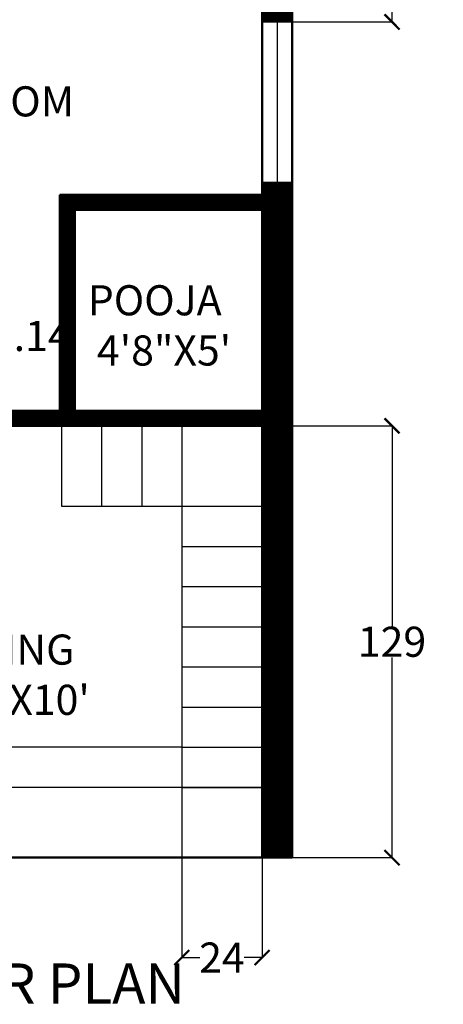
# Model space of a CAD drawing. Units: inches. Extents: x 104 to 466, y -74 to 547.
# Tile 2 of 4: x 320 to 447, y -74 to 220. Entities that reach past the tile are written whole.
import ezdxf

# ---------------------------------------------------------------- set-up
doc = ezdxf.new("R2010")
doc.units = ezdxf.units.IN
doc.header["$MEASUREMENT"] = 0
for name, color, linetype, lineweight in [('A-ANNO-DIMS', 2, 'Continuous', 18), ('A-ANNO-TEXT', 7, 'Continuous', 35), ('A-AREA-IDEN', 7, 'Continuous', 25), ('A-FLOR-STRS', 7, 'Continuous', 25), ('A-GLAZ', 4, 'Continuous', 25), ('A-WALL', 7, 'Continuous', 50), ('A-WALL-PATT', 8, 'Continuous', 13)]:
    doc.layers.add(name, color=color, linetype=linetype, lineweight=lineweight)
doc.styles.get("Standard").update_dxf_attribs({"font": 'arial.ttf'})
doc.dimstyles.get("Standard").update_dxf_attribs({"dimtxt": 9, "dimasz": 4.5, "dimexe": 0.18, "dimexo": 0.0625, "dimgap": 0.09, "dimtad": 0, "dimtih": 1, "dimtoh": 1, "dimdec": 1, "dimzin": 0, "dimdsep": 46, "dimlunit": 4, "dimtxsty": 'Standard', "dimblk": 'ARCHTICK', "dimcen": 0.09, "dimadec": 0, "dimazin": 0, "dimtfac": 1, "dimtdec": 1, "dimtofl": 0, "dimtmove": 0, "dimatfit": 3, "dimfxl": 1, "dimtolj": 1, "dimtzin": 0, "dimarcsym": 0})

# ---------------------------------------------------------------- blocks, each defined once
blk = doc.blocks.new('WINDOW-48IN')
for p, q in [((0, 48), (9, 48)), ((0, 0), (0, 48)), ((4.5, 48), (4.5, 0)), ((9, 48), (9, 0)), ((9, 0), (0, 0))]:
    blk.add_line(p, q)
blk = doc.blocks.new('_ArchTick')
at = {"color": 0, "linetype": 'ByBlock', "const_width": 0.15}
blk.add_lwpolyline([(-0.5, -0.5), (0.5, 0.5)], dxfattribs=at)
blk = doc.blocks.new('*D25')
at = {"layer": 'A-ANNO-DIMS', "color": 0, "lineweight": -2, "transparency": 16777216}
for p, q in [((401.65, 292.54), (431.61, 292.54)), ((431.43, 292.54), (431.43, 260.56)), ((431.43, 219.21), (431.43, 251.19)), ((401.65, 219.21), (431.61, 219.21))]:
    blk.add_line(p, q, dxfattribs=at)
at = {"layer": 'Defpoints', "color": 0, "transparency": 16777216}
for p in [(401.58, 292.54), (401.58, 219.21), (431.43, 219.21)]:
    blk.add_point(p, dxfattribs=at)
at = {"layer": 'A-ANNO-DIMS', "color": 0, "lineweight": -2, "transparency": 16777216, "xscale": 4.5, "yscale": 4.5, "zscale": 4.5}
for p, rotation in [((431.43, 292.54), 90), ((431.43, 219.21), 270)]:
    blk.add_blockref('_ArchTick', p, dxfattribs=dict(at, rotation=rotation))
at = {"layer": 'A-ANNO-DIMS', "color": 0, "transparency": 16777216, "insert": (431.43, 255.88), "char_height": 9, "attachment_point": 5}
blk.add_mtext('\\A1;73.33', dxfattribs=at)
blk = doc.blocks.new('*D28')
at = {"layer": 'A-ANNO-DIMS', "color": 0, "lineweight": -2, "transparency": 16777216}
for p, q in [((392.65, 98.54), (431.61, 98.54)), ((431.43, 98.54), (431.43, 38.73)), ((431.43, -30.46), (431.43, 29.36)), ((401.65, -30.46), (431.61, -30.46))]:
    blk.add_line(p, q, dxfattribs=at)
at = {"layer": 'Defpoints', "color": 0, "transparency": 16777216}
for p in [(392.58, 98.54), (431.43, 98.54), (401.58, -30.46)]:
    blk.add_point(p, dxfattribs=at)
at = {"layer": 'A-ANNO-DIMS', "color": 0, "lineweight": -2, "transparency": 16777216, "xscale": 4.5, "yscale": 4.5, "zscale": 4.5}
for p, rotation in [((431.43, 98.54), 90), ((431.43, -30.46), 270)]:
    blk.add_blockref('_ArchTick', p, dxfattribs=dict(at, rotation=rotation))
at = {"layer": 'A-ANNO-DIMS', "color": 0, "transparency": 16777216, "insert": (431.43, 34.04), "char_height": 9, "attachment_point": 5}
blk.add_mtext('\\A1;129', dxfattribs=at)
blk = doc.blocks.new('*D29')
at = {"layer": 'A-ANNO-DIMS', "color": 0, "lineweight": -2, "transparency": 16777216}
for p, q in [((368.58, -9.52), (368.58, -60.49)), ((392.58, -9.52), (392.58, -60.49)), ((368.58, -60.31), (373.99, -60.31)), ((392.58, -60.31), (387.18, -60.31))]:
    blk.add_line(p, q, dxfattribs=at)
at = {"layer": 'Defpoints', "color": 0, "transparency": 16777216}
for p in [(368.58, -9.46), (392.58, -9.46), (368.58, -60.31)]:
    blk.add_point(p, dxfattribs=at)
at = {"layer": 'A-ANNO-DIMS', "color": 0, "lineweight": -2, "transparency": 16777216, "xscale": 4.5, "yscale": 4.5, "zscale": 4.5, "rotation": 180}
blk.add_blockref('_ArchTick', (368.58, -60.31), dxfattribs=at)
at = {"layer": 'A-ANNO-DIMS', "color": 0, "lineweight": -2, "transparency": 16777216, "xscale": 4.5, "yscale": 4.5, "zscale": 4.5}
blk.add_blockref('_ArchTick', (392.58, -60.31), dxfattribs=at)
at = {"layer": 'A-ANNO-DIMS', "color": 0, "transparency": 16777216, "insert": (380.58, -60.31), "char_height": 9, "attachment_point": 5}
blk.add_mtext('\\A1;24', dxfattribs=at)
blk = doc.blocks.new('*D30')
at = {"layer": 'A-ANNO-DIMS', "color": 0, "lineweight": -2, "transparency": 16777216}
for p, q in [((368.52, 2.54), (129.05, 2.54)), ((129.23, 2.54), (129.23, 1.15)), ((129.23, -9.46), (129.23, -8.06)), ((368.52, -9.46), (129.05, -9.46))]:
    blk.add_line(p, q, dxfattribs=at)
at = {"layer": 'Defpoints', "color": 0, "transparency": 16777216}
for p in [(129.23, 2.54), (368.58, 2.54), (368.58, -9.46)]:
    blk.add_point(p, dxfattribs=at)
at = {"layer": 'A-ANNO-DIMS', "color": 0, "lineweight": -2, "transparency": 16777216, "xscale": 4.5, "yscale": 4.5, "zscale": 4.5}
for p, rotation in [((129.23, 2.54), 90), ((129.23, -9.46), 270)]:
    blk.add_blockref('_ArchTick', p, dxfattribs=dict(at, rotation=rotation))
at = {"layer": 'A-ANNO-DIMS', "color": 0, "transparency": 16777216, "insert": (129.23, -3.46), "char_height": 9, "attachment_point": 5}
blk.add_mtext('\\A1;12', dxfattribs=at)
blk = doc.blocks.new('*D36')
at = {"layer": 'A-ANNO-DIMS', "color": 0, "lineweight": -2, "transparency": 16777216}
for p, q in [((392.52, -9.46), (129.05, -9.46)), ((129.23, -9.46), (129.23, -15.35)), ((129.23, -30.46), (129.23, -24.56)), ((392.52, -30.46), (129.05, -30.46))]:
    blk.add_line(p, q, dxfattribs=at)
at = {"layer": 'Defpoints', "color": 0, "transparency": 16777216}
for p in [(392.58, -9.46), (129.23, -30.46), (392.58, -30.46)]:
    blk.add_point(p, dxfattribs=at)
at = {"layer": 'A-ANNO-DIMS', "color": 0, "lineweight": -2, "transparency": 16777216, "xscale": 4.5, "yscale": 4.5, "zscale": 4.5}
for p, rotation in [((129.23, -9.46), 90), ((129.23, -30.46), 270)]:
    blk.add_blockref('_ArchTick', p, dxfattribs=dict(at, rotation=rotation))
at = {"layer": 'A-ANNO-DIMS', "color": 0, "transparency": 16777216, "insert": (129.23, -19.96), "char_height": 9, "attachment_point": 5}
blk.add_mtext('\\A1;21', dxfattribs=at)
blk = doc.blocks.new('*D67')
at = {"layer": 'A-ANNO-DIMS', "color": 0, "lineweight": -2, "transparency": 16777216}
for p, q in [((292.06, 125.4), (281.76, 117.02)), ((296.56, 125.4), (292.06, 125.4)), ((264.49, 103.04), (264.67, 103.04)), ((264.58, 102.95), (264.58, 103.13))]:
    blk.add_line(p, q, dxfattribs=at)
at = {"layer": 'Defpoints', "color": 0, "transparency": 16777216}
for p in [(281.76, 117.02), (264.58, 103.04)]:
    blk.add_point(p, dxfattribs=at)
at = {"layer": 'A-ANNO-DIMS', "color": 0, "lineweight": -2, "transparency": 16777216, "xscale": 4.5, "yscale": 4.5, "zscale": 4.5, "rotation": 219.1362079065188}
blk.add_blockref('_ArchTick', (281.76, 117.02), dxfattribs=at)
at = {"layer": 'A-ANNO-DIMS', "color": 0, "transparency": 16777216, "insert": (316.12, 125.4), "char_height": 9, "attachment_point": 5}
blk.add_mtext('\\A1;R22.14', dxfattribs=at)

msp = doc.modelspace()

# ---------------------------------------------------------------- hatches: boundary and pattern name
at = {"layer": 'A-WALL-PATT'}
h = msp.add_hatch(dxfattribs=at)
h.set_pattern_fill('ANSI31', color=256)
h.set_pattern_definition([(45, (-366.28003, -301.99136), (-0.088388348, 0.088388348), [])])
h.paths.add_polyline_path([(401.5842, 137.0851), (401.5842, 171.2112), (392.5842, 171.2112), (392.5842, 167.545), (332.0842, 167.545), (332.0842, 137.0851), (332.0842, 103.045), (312.5842, 103.045), (312.5842, 98.545), (392.5842, 98.545), (392.5842, -9.455), (392.5842, -30.455), (401.5842, -30.455), (401.5842, 31.361)])
h.paths.add_polyline_path([(392.5842, 103.045), (336.5842, 103.045), (336.5842, 137.0851), (336.5842, 163.045), (392.5842, 163.045), (392.5842, 137.0851)], flags=16)
h.paths.add_polyline_path([(401.5842, 292.5416), (392.5842, 292.5416), (392.5842, 227.545), (248.5842, 227.545), (248.5842, 232.045), (244.0842, 232.045), (244.0842, 223.045), (248.5842, 223.045), (392.5842, 223.045), (392.5842, 219.2112), (401.5842, 219.2112)])
h.paths.add_polyline_path([(401.5842, 388.2533), (392.5842, 388.2533), (392.5842, 370.045), (340.5842, 370.045), (340.5842, 369.865, -0.03576944), (340.8936, 365.545), (392.5842, 365.545), (392.5842, 340.5416), (401.5842, 340.5416)], flags=17)
h.paths.add_polyline_path([(401.5842, 453.4958), (392.5842, 453.4958), (392.5842, 438.045), (310.5842, 438.045), (310.5842, 467.545), (306.0842, 467.545), (306.0842, 370.045), (208.837, 370.045, -0.03088397), (209.1152, 365.545), (244.0842, 365.545), (244.0842, 274.587, -0.0265002), (248.5842, 274.3483), (248.5842, 365.545), (306.0842, 365.545), (310.5842, 365.545), (310.5842, 370.045), (310.5842, 433.545), (392.5842, 433.545), (392.5842, 424.2533), (401.5842, 424.2533)])
h.paths.add_polyline_path([(168.0842, 365.545), (172.5842, 365.545), (172.5842, 370.045), (168.0842, 370.045), (168.0842, 414.671), (159.0842, 414.671), (159.0842, 214.5244), (168.0842, 214.5244)])
h.paths.add_polyline_path([(168.0842, 98.545), (224.0842, 98.545), (224.0842, 103.045), (168.0842, 103.045), (168.0842, 137.0851), (168.0842, 166.5244), (159.0842, 166.5244), (159.0842, 137.0851), (159.0842, 43.0309), (159.0842, -30.455), (168.0842, -30.455), (177.7316, -30.455), (177.7316, -21.455), (168.0842, -21.455), (168.0842, 35.9487)])
h.paths.add_polyline_path([(264.5842, -21.455), (264.5842, 98.545), (264.5842, 103.045), (260.3643, 103.045, -0.03109877), (260.0842, 98.545), (260.0842, -21.455), (248.5842, -21.455), (213.7316, -21.455), (213.7316, -30.455), (248.5842, -30.455), (264.5842, -30.455)])
h.paths.add_polyline_path([(401.5842, 511.045), (159.0842, 511.045), (159.0842, 462.671), (168.0842, 462.671), (168.0842, 502.045), (306.0842, 502.045), (306.0842, 497.545), (310.5842, 497.545), (310.5842, 502.045), (392.5842, 502.045), (392.5842, 489.4958), (401.5842, 489.4958)])

# ---------------------------------------------------------------- linework, layer by layer
at = {"layer": 'A-FLOR-STRS'}
for p, q in [((332.5842, 98.545), (332.5842, 74.545)), ((344.5842, 98.545), (344.5842, 74.545)), ((356.5842, 98.545), (356.5842, 74.545)), ((356.5842, 98.545), (356.5842, 74.545)), ((368.5842, 98.545), (368.5842, -9.455)), ((332.5842, 74.545), (392.5842, 74.545)), ((368.5842, 62.545), (392.5842, 62.545)), ((368.5842, 50.545), (392.5842, 50.545)), ((368.5842, 38.545), (392.5842, 38.545)), ((368.5842, 26.545), (392.5842, 26.545)), ((368.5842, 14.545), (392.5842, 14.545)), ((368.5842, 2.545), (392.5842, 2.545)), ((368.5842, -9.455), (392.5842, -9.455))]:
    msp.add_line(p, q, dxfattribs=at)
at = {"layer": 'A-WALL'}
for p, q in [((401.5842, 511.045), (401.5842, 137.0851)), ((392.5842, 223.045), (392.5842, 167.545)), ((332.0842, 167.545), (392.5842, 167.545)), ((332.0842, 167.545), (332.0842, 137.0851)), ((336.5842, 163.045), (336.5842, 137.0851)), ((336.5842, 163.045), (392.5842, 163.045)), ((392.5842, 163.045), (392.5842, 137.0851)), ((332.0842, 137.0851), (332.0842, 103.045)), ((336.5842, 137.0851), (336.5842, 103.045)), ((392.5842, 137.0851), (392.5842, 103.045)), ((401.5842, 137.0851), (401.5842, 31.361)), ((312.5842, 103.045), (332.0842, 103.045)), ((336.5842, 103.045), (392.5842, 103.045)), ((312.5842, 98.545), (392.5842, 98.545)), ((392.5842, 98.545), (392.5842, -9.455)), ((401.5842, 31.361), (401.5842, -30.455)), ((392.5842, -9.455), (392.5842, -30.455)), ((248.5842, -30.455), (392.5842, -30.455)), ((392.5842, -30.455), (401.5842, -30.455))]:
    msp.add_line(p, q, dxfattribs=at)

# ---------------------------------------------------------------- block references
at = {"layer": 'A-GLAZ'}
msp.add_blockref('WINDOW-48IN', (392.584, 171.211), dxfattribs=at)

# ---------------------------------------------------------------- texts
at = {"layer": 'A-ANNO-TEXT', "insert": (199.8176, -62.0596), "char_height": 12, "attachment_point": 1}
msp.add_mtext_dynamic_manual_height_columns('GROUND FLOOR PLAN', width=401.09946, gutter_width=1, heights=[0], dxfattribs=at)
at = {"layer": 'A-AREA-IDEN', "char_height": 9, "attachment_point": 1}
for s, insert in [(' HALL CUM LIVING ROOM\\P              18\'8"X10\'', (194.7177, 199.983)), ('  POOJA \\P   4\'8"X5\'', (334.954, 140.5599)), ('PARKING\\P 10\'8"X10\'', (284.5647, 36.1976))]:
    msp.add_mtext_dynamic_manual_height_columns(s, width=401.09946, gutter_width=1, heights=[0], dxfattribs=dict(at, insert=insert))

# ---------------------------------------------------------------- dimensions: what is measured, and where the dimension line sits
at = {"layer": 'A-ANNO-DIMS'}
for base, p1, p2, override, picture, middle in [((431.4342, 219.2112), (401.5842, 292.5416), (401.5842, 219.2112), {"dimdec": 2, "dimlfac": 1, "dimrnd": 0, "dimzin": 0, "dimdsep": 46, "dimlunit": 2}, '*D25', (431.4342, 255.8764)), ((431.4342, 98.545), (401.5842, -30.455), (392.5842, 98.545), {"dimdec": 0, "dimlfac": 1, "dimrnd": 0, "dimzin": 0, "dimdsep": 46, "dimlunit": 2}, '*D28', (431.4342, 34.045)), ((129.2342, 2.545), (368.5842, -9.455), (368.5842, 2.545), {"dimdec": 0, "dimlfac": 1, "dimrnd": 0, "dimzin": 0, "dimdsep": 46, "dimlunit": 2}, '*D30', (129.2342, -3.455)), ((129.2342, -30.455), (392.5842, -9.455), (392.5842, -30.455), {"dimdec": 0, "dimlfac": 1, "dimrnd": 0, "dimzin": 0, "dimdsep": 46, "dimlunit": 2}, '*D36', (129.2342, -19.955))]:
    dim = msp.add_linear_dim(base=base, p1=p1, p2=p2, angle=90, dimstyle='Standard', override=override, dxfattribs=at)
    dim.commit()
    dim.dimension.update_dxf_attribs({"geometry": picture, "text_midpoint": middle})
dim = msp.add_radius_dim(center=(264.5842, 103.045), mpoint=(281.7571, 117.0191), dimstyle='Standard', override={"dimdec": 2, "dimlfac": 1, "dimrnd": 0, "dimzin": 0, "dimdsep": 46, "dimlunit": 2}, dxfattribs=at)
dim.commit()
dim.dimension.update_dxf_attribs({"geometry": '*D67', "text_midpoint": (316.1242, 125.4035), "dimtype": 164})
dim = msp.add_linear_dim(base=(368.5842, -60.305), p1=(392.5842, -9.455), p2=(368.5842, -9.455), dimstyle='Standard', override={"dimdec": 0, "dimlfac": 1, "dimrnd": 0, "dimzin": 0, "dimdsep": 46, "dimlunit": 2}, dxfattribs=at)
dim.commit()
dim.dimension.update_dxf_attribs({"geometry": '*D29', "text_midpoint": (380.5842, -60.305)})

doc.saveas('drawing.dxf')
